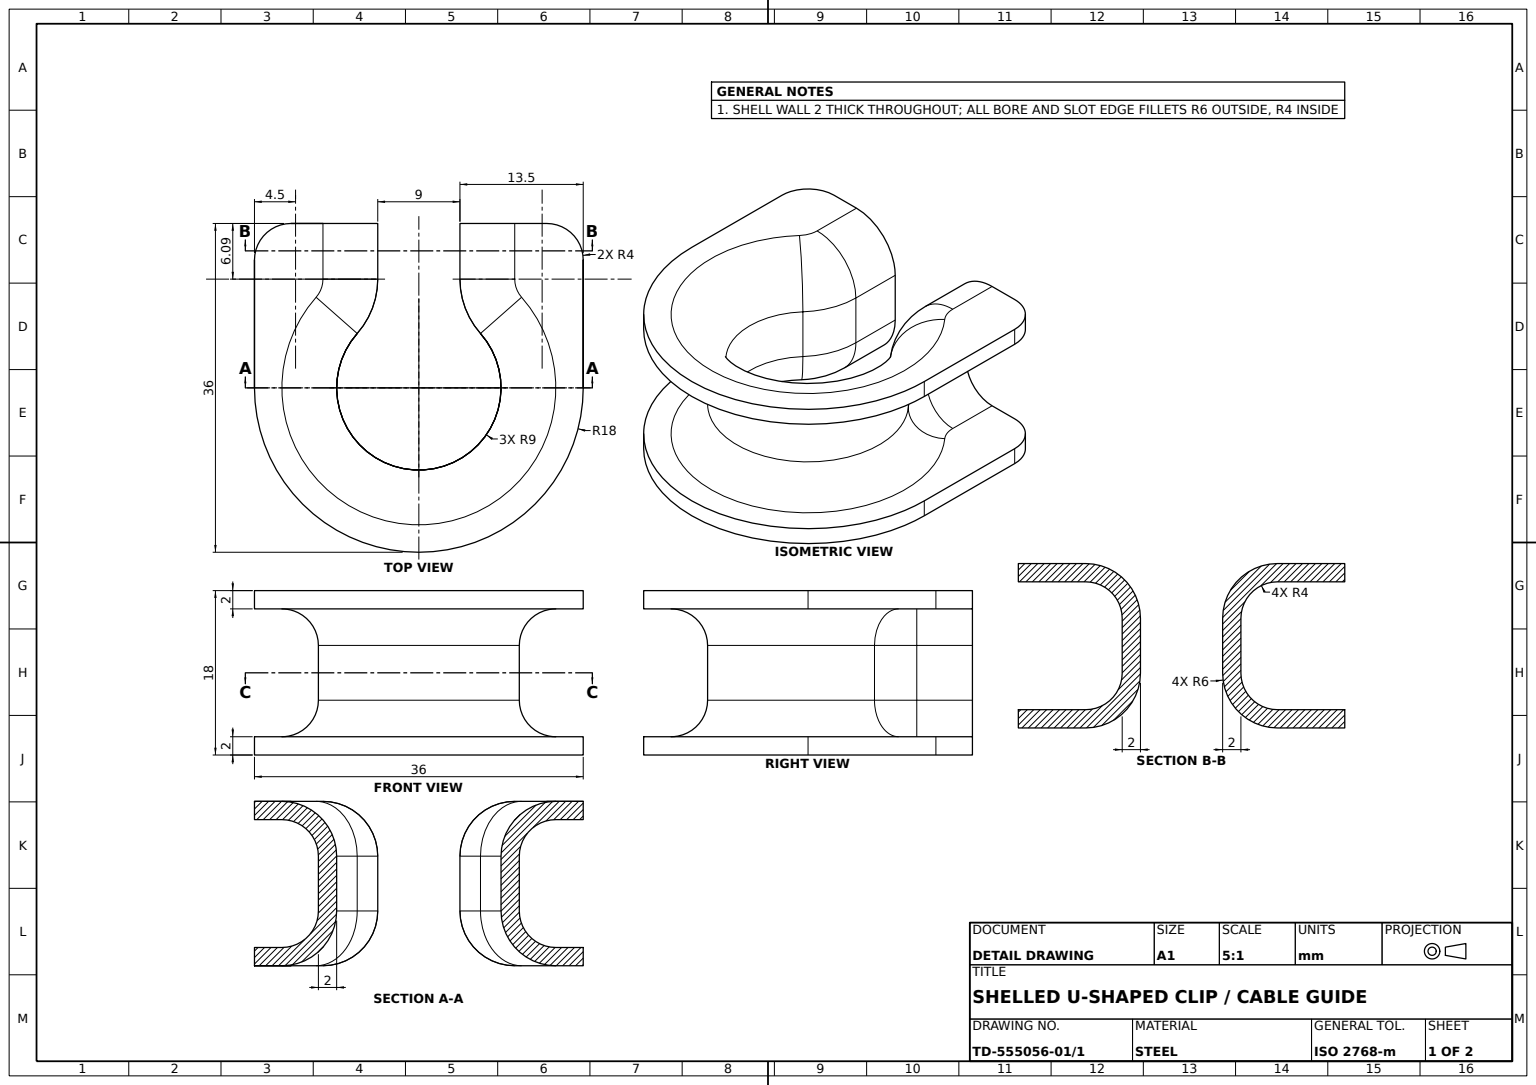
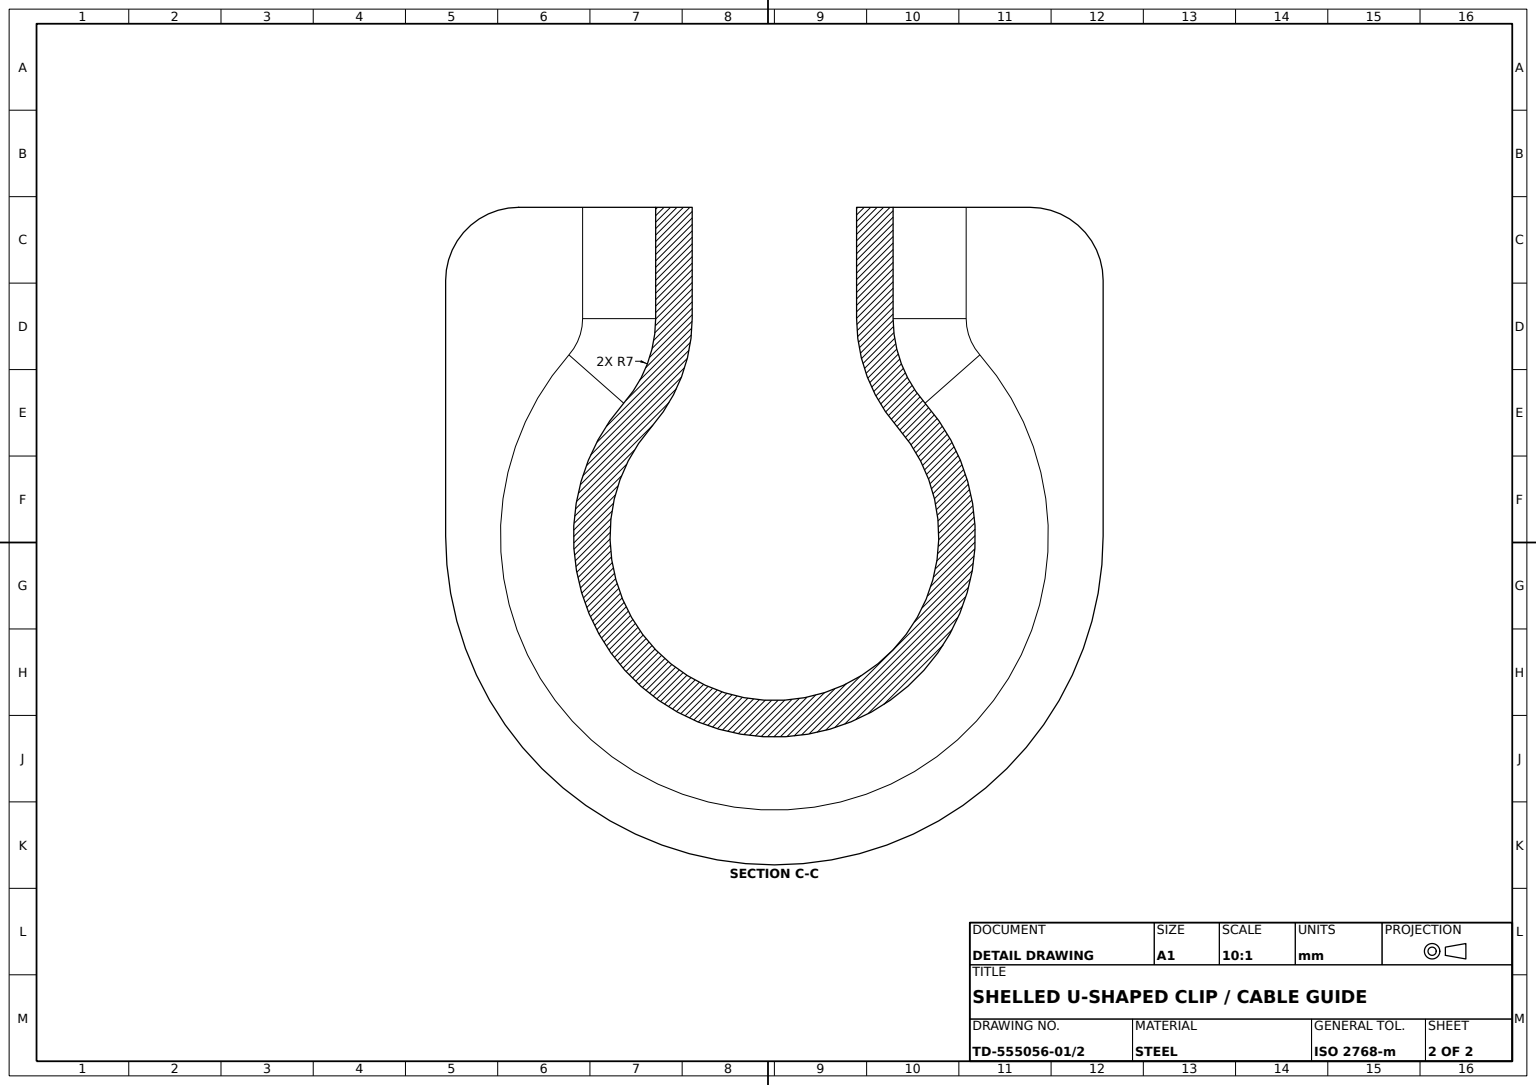
SolidWorks part; units mm, degrees
material "Plain Carbon Steel"
ref_plane "Front Plane" through (0, 0, 0) normal (0, 0, 1) x (1, 0, 0)
ref_plane "Top Plane" through (0, 0, 0) normal (0, 1, 0) x (1, 0, 0)
ref_plane "Right Plane" through (0, 0, 0) normal (1, 0, 0) x (0, 0, -1)
sketch "Clip Profile Sketch" plane through (0, 0, 0) normal (0, 1, 0) x (1, 0, 0)
  line L0 (-14, 18) -> (-4.5, 18)
  line L1 (0, 22.024) -> (0, 0) construction
  line L2 (-4.5, 18) -> (-4.5, 11.9059)
  line L3 (4.5, 18) -> (4.5, 11.9059)
  line L4 (4.5, 18) -> (14, 18)
  line L5 (18, 14) -> (18, 0)
  line L6 (-18, 14) -> (-18, 0)
  arc A0 (-6.75, 5.9529) -> (6.75, 5.9529) centre (0, 0) ccw
  arc A1 (-4.5, 11.9059) -> (-6.75, 5.9529) centre (-13.5, 11.9059) cw
  arc A2 (4.5, 11.9059) -> (6.75, 5.9529) centre (13.5, 11.9059) ccw
  arc A3 (-18, 0) -> (18, 0) centre (0, 0) ccw
  arc A4 (18, 14) -> (14, 18) centre (14, 14) ccw
  arc A5 (-14, 18) -> (-18, 14) centre (-14, 14) ccw
  point P17 (18, 18)
  dimension "D1" = 18
  dimension "D3" = 9
  dimension "D6" = 36
  dimension "D7" = 4
  dimension "D2" = 18
  dimension "D4" = 4.5
  dimension "D5" = 18
extrude "Clip Body Extrude 18mm" add sketch "Clip Profile Sketch" along normal mid plane 18
fillet "Edge Fillets R6" radius 6 10 edges at (4.5, -9, -14.9529) (5.0813, -9, -8.7239) (-4.5, -9, -14.9529) (-5.0813, -9, -8.7239) (4.5, 9, -14.9529) (-4.5, 9, -14.9529) (-5.0813, 9, -8.7239) (0, 9, 9) (0, -9, 9) (5.0813, 9, -8.7239)
shell "Shell Wall 2mm" thickness 2
